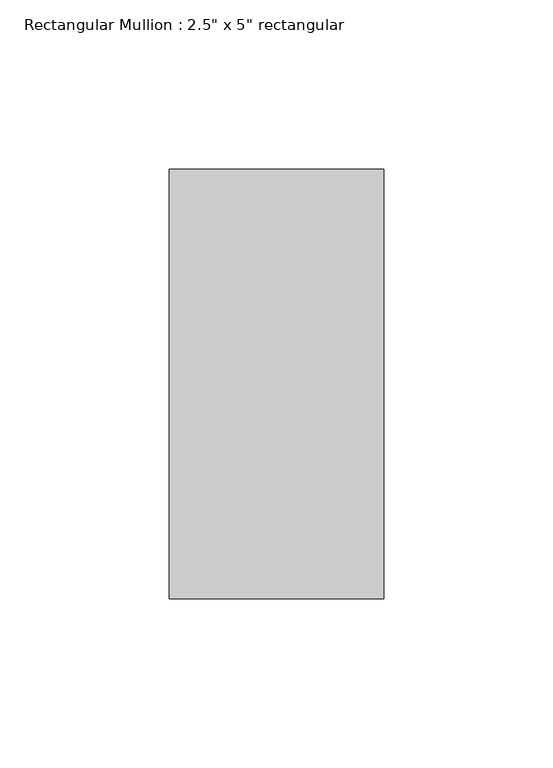
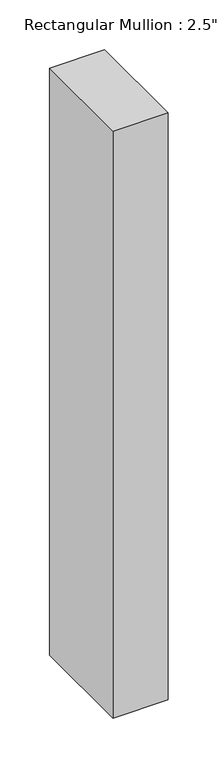
"""IFC4 building model written with IfcOpenShell, lengths in millimetres: member geometry."""

from ifc_helpers import new_model, si_unit, frame, origin, place, context, project, spatial, polyline, outline, extrude, source, transform, mapped, element, save


def member_7007ad49(model_context):
    return source(origin(), model_context, "Body", "SweptSolid", [
        extrude(outline(polyline([(0.0, 63.5), (0.0, -63.5), (-63.5, -63.5), (-63.5, 63.5), (0.0, 63.5)])), frame((0.0, 0.0, -717.55), z_axis=(0.0, 0.0, 1.0), x_axis=(1.0, 0.0, 0.0)), (0.0, 0.0, 1.0), 717.55),
    ])


if __name__ == "__main__":
    model = new_model("IFC4")
    model_context = context("Model", 3, world=origin())
    ifc_project = project(units=[si_unit("LENGTHUNIT", "METRE", prefix="MILLI")], contexts=[model_context])
    site = spatial("IfcSite", under=ifc_project)
    building = spatial("IfcBuilding", under=site)
    placement = place(None, origin())
    member_shape = member_7007ad49(model_context)
    element("IfcMember", 1, ObjectType="Rectangular Mullion : 2.5\" x 5\" rectangular", at=placement, inside=building, context=model_context, shape_type="MappedRepresentation", body=[
        mapped(member_shape, transform((0.0, 0.0, 0.0), x_axis=(1.0, 0.0, 0.0), y_axis=(0.0, 1.0, 0.0), z_axis=(0.0, 0.0, 1.0))),
    ])
    save(model, "model.ifc")

# Revit data of these elements
# Type "Rectangular Mullion : 2.5\" x 5\" rectangular"
#   built-in parameter 1007304 = 0.416667 (stored number, unit not read)
#   built-in parameter 1007301 = 0.104167 (stored number, unit not read)
#   built-in parameter 1007300 = 0.104167 (stored number, unit not read)
